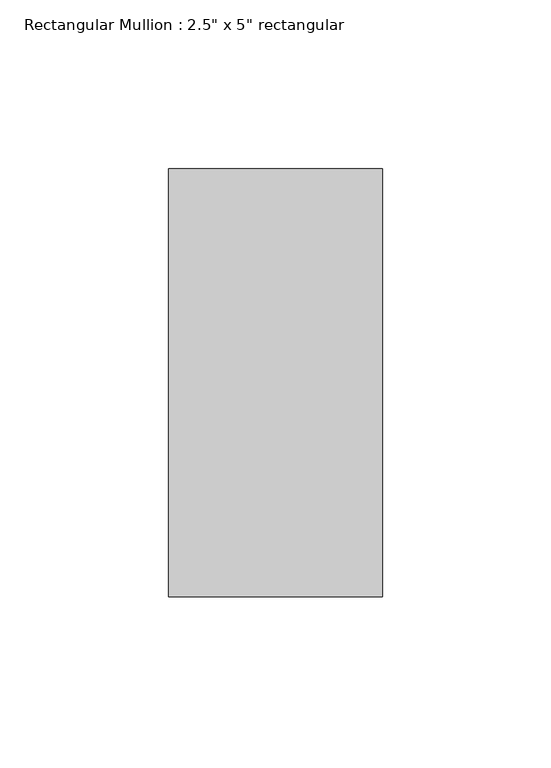
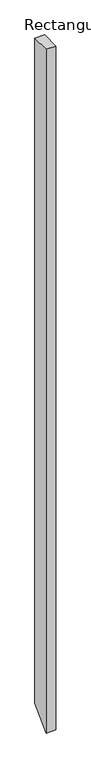
"""IFC4 building model written with IfcOpenShell, lengths in millimetres: member geometry."""

from ifc_helpers import new_model, si_unit, frame, origin, place, context, project, spatial, polyline, outline, extrude, source, transform, mapped, element, save


def member_fc2d78a3(model_context):
    return source(origin(), model_context, "Body", "SweptSolid", [
        extrude(outline(polyline([(-63.5, 0.0), (63.5, 0.0), (63.5, -4575.3282426), (-63.5, -4702.3282426), (-63.5, 0.0)])), frame((-63.5, 0.0, 0.0), z_axis=(1.0, 0.0, 0.0), x_axis=(0.0, 1.0, 0.0)), (0.0, 0.0, 1.0), 63.5),
    ])


if __name__ == "__main__":
    model = new_model("IFC4")
    model_context = context("Model", 3, world=origin())
    ifc_project = project(units=[si_unit("LENGTHUNIT", "METRE", prefix="MILLI")], contexts=[model_context])
    site = spatial("IfcSite", under=ifc_project)
    building = spatial("IfcBuilding", under=site)
    placement = place(None, origin())
    member_shape = member_fc2d78a3(model_context)
    element("IfcMember", 1, ObjectType="Rectangular Mullion : 2.5\" x 5\" rectangular", at=placement, inside=building, context=model_context, shape_type="MappedRepresentation", body=[
        mapped(member_shape, transform((0.0, 0.0, 0.0), x_axis=(1.0, 0.0, 0.0), y_axis=(0.0, 1.0, 0.0), z_axis=(0.0, 0.0, 1.0))),
    ])
    save(model, "model.ifc")

# Revit data of these elements
# Type "Rectangular Mullion : 2.5\" x 5\" rectangular"
#   built-in parameter 1007304 = 0.416667 (stored number, unit not read)
#   built-in parameter 1007301 = 0.104167 (stored number, unit not read)
#   built-in parameter 1007300 = 0.104167 (stored number, unit not read)
# Element 1 (IfcMember, "Rectangular Mullion : 2.5\" x 5\" rectangular")
#   Materials on its faces: "Aluminum"
# Materials
#   "Aluminum": class "Metal", colour RGB 247 247 247, transparency 0, Description = "Aluminum 6061", Cost = 0
